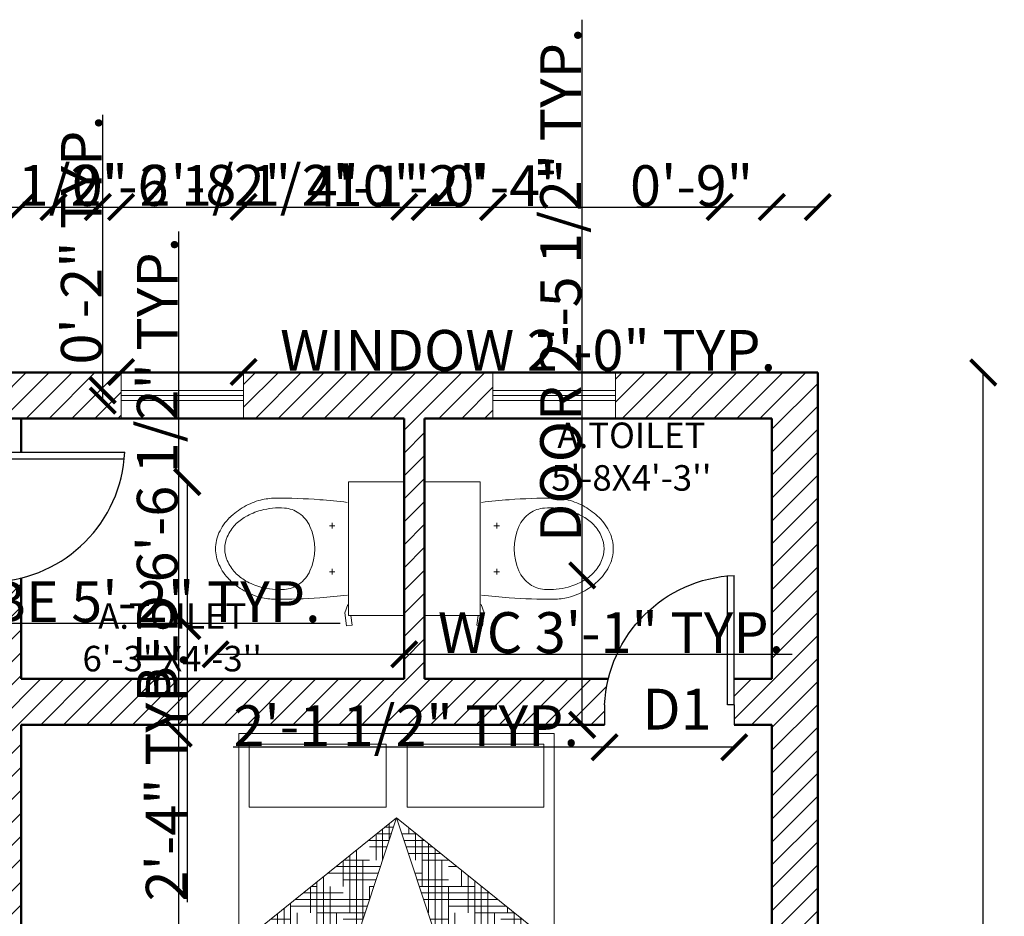
# Model space of a CAD drawing. Units: inches. Extents: x 1385 to 1778, y 1343 to 2100.
# Tile 6 of 6: x 1571 to 1764, y 1924 to 2100. Entities that reach past the tile are written whole.
import ezdxf

# ---------------------------------------------------------------- set-up
doc = ezdxf.new("R2010")
doc.units = ezdxf.units.IN
for name, color, linetype, lineweight in [('A-ANNO-DIMS', 2, 'Continuous', 18), ('A-ANNO-TEXT', 7, 'Continuous', 25), ('A-AREA-IDEN', 7, 'Continuous', 25), ('A-FLOR-FIXT', 9, 'Continuous', 18), ('A-FURN', 8, 'Continuous', 18), ('A-WALL-PATT', 8, 'Continuous', 13), ('Door', 150, 'Continuous', 25), ('Wall', 7, 'Continuous', 50), ('Windows', 140, 'Continuous', 18)]:
    doc.layers.add(name, color=color, linetype=linetype, lineweight=lineweight)
doc.styles.get("Standard").update_dxf_attribs({"font": 'arial.ttf'})
doc.dimstyles.get("Standard").update_dxf_attribs({"dimtxt": 8, "dimasz": 5, "dimexe": 0.18, "dimexo": 0.0625, "dimgap": 0.09, "dimtad": 1, "dimdec": 1, "dimzin": 0, "dimdsep": 46, "dimlunit": 4, "dimtxsty": 'Standard', "dimblk": 'ARCHTICK', "dimcen": 0.09, "dimse1": 1, "dimse2": 1, "dimadec": 0, "dimazin": 0, "dimtfac": 1, "dimtdec": 1, "dimtofl": 0, "dimtmove": 0, "dimatfit": 3, "dimfxl": 1, "dimtolj": 1, "dimtzin": 0, "dimarcsym": 0})

# ---------------------------------------------------------------- blocks, each defined once
blk = doc.blocks.new('AP0B05')
for p, q in [((35, 100), (35, 880)), ((75, 100), (75, 878.9)), ((35, 100), (35, -20)), ((815, 100), (815, -20))]:
    blk.add_line(p, q)
blk.add_lwpolyline([(35, 100), (75, 100)])
blk.add_arc((-2.4, 62.6), 818.3, 2.62122, 87.37878)
blk = doc.blocks.new('toilet-1')
at = {"color": 0, "linetype": 'ByBlock'}
for p, q in [((-0.23, -0.02), (-0.23, -0.2116)), ((0.23, -0.02), (-0.23, -0.02)), ((0.23, -0.02), (0.23, -0.2116)), ((0.2633, -0.1997), (0.23, -0.2044)), ((0.266, -0.2187), (0.2633, -0.1997)), ((-0.23, -0.2116), (0.23, -0.2116)), ((0.1917, -0.2144), (0.2206, -0.225)), ((0.2206, -0.225), (0.266, -0.2187)), ((-0.0889, -0.2683), (-0.0697, -0.2683)), ((-0.0793, -0.2587), (-0.0793, -0.2778)), ((0.0889, -0.2683), (0.0698, -0.2683)), ((0.0794, -0.2587), (0.0794, -0.2778)), ((0, -0.6382), (0, -0.6382))]:
    blk.add_line(p, q, dxfattribs=at)
for centre, radius, start, end in [((3.5272, -0.6239), 3.7093, 173.6925, 175.1593), ((-3.527, -0.624), 3.7093, 4.8413, 6.3171), ((1.7368, -0.4519), 1.9109, 175.7698, 180.3758), ((0, -0.5169), 0.1884, 66.0939, 113.9061), ((-1.7366, -0.4519), 1.9109, 359.6242, 4.2302), ((-0.0312, -0.4465), 0.1114, 113.8997, 145.1485), ((0.0312, -0.4465), 0.1114, 34.8515, 66.1003), ((-0.0408, -0.4398), 0.0996, 145.1497, 175.881), ((0.0409, -0.4398), 0.0996, 4.119, 34.8503), ((0.0981, -0.4497), 0.2389, 175.8862, 195.5931), ((-0.098, -0.4497), 0.2389, 344.4069, 4.1138), ((0.0353, -0.463), 0.2093, 180.3747, 194.3375), ((-0.0351, -0.463), 0.2093, 345.6614, 359.6243), ((0.055, -0.458), 0.2297, 194.3353, 209.622), ((0.0961, -0.4503), 0.2369, 195.5969, 209.3771), ((-0.096, -0.4503), 0.2369, 330.6229, 344.4031), ((-0.0548, -0.458), 0.2297, 330.3788, 345.6655), ((0.0647, -0.4524), 0.2409, 209.6273, 224.5489), ((0.0232, -0.4913), 0.1532, 209.3871, 226.5438), ((-0.0231, -0.4913), 0.1532, 313.4562, 330.6129), ((-0.0645, -0.4524), 0.2409, 315.4504, 330.372), ((0.0152, -0.4997), 0.1416, 226.5501, 246.5527), ((-0.0151, -0.4997), 0.1416, 293.4473, 313.4499), ((0.0178, -0.4986), 0.1751, 224.552, 245.714), ((0, -0.5347), 0.1034, 246.5493, 270.0042), ((0, -0.5347), 0.1034, 269.9958, 293.4507), ((-0.0176, -0.4986), 0.1751, 294.2865, 315.4485), ((0.0004, -0.538), 0.132, 245.5845, 269.8782), ((-0.0002, -0.538), 0.132, 270.1216, 294.4153)]:
    blk.add_arc(centre, radius, start, end, dxfattribs=at)
blk = doc.blocks.new('*X10')
at = {"color": 0}
for p, q in [((20.25, 14.8125), (20.2772, 14.8125)), ((20.1739, 14.75), (20.2772, 14.75)), ((20.1875, 14.75), (20.1875, 14.7669)), ((20.199, 14.7812), (20.2772, 14.7812)), ((20.25, 14.3194), (20.25, 14.75)), ((20.1487, 14.7188), (20.2772, 14.7188)), ((20.1562, 14.625), (20.1562, 14.7281)), ((20.0984, 14.6562), (20.125, 14.6562)), ((20.1236, 14.6875), (20.25, 14.6875)), ((20.125, 14.5), (20.125, 14.6893)), ((20.0625, 14.2573), (20.0625, 14.6116)), ((20.0938, 14.375), (20.0938, 14.6504)), ((20.2188, 14.3091), (20.2188, 14.625)), ((20.25, 14.625), (20.2772, 14.625)), ((20.023, 14.5625), (20.2772, 14.5625)), ((20.0312, 14.2469), (20.0312, 14.5727)), ((20.125, 14.5938), (20.2772, 14.5938)), ((19.9979, 14.5312), (20.2772, 14.5312)), ((19.9476, 14.4688), (20.125, 14.4688)), ((19.9727, 14.5), (20.25, 14.5)), ((20, 14.2366), (20, 14.5)), ((20.1875, 14.2987), (20.1875, 14.5)), ((19.9062, 14.375), (19.9062, 14.4174)), ((19.9225, 14.4375), (20, 14.4375)), ((20.25, 14.4375), (20.2772, 14.4375)), ((19.875, 14.25), (19.875, 14.3785)), ((19.9688, 14.2262), (19.9688, 14.375)), ((20, 14.375), (20.2772, 14.375)), ((20.125, 14.4062), (20.2772, 14.4062)), ((20.1562, 14.2884), (20.1562, 14.375)), ((19.8438, 14.1848), (19.8438, 14.3397)), ((19.875, 14.3438), (20.2772, 14.3438)), ((19.7967, 14.2812), (20.125, 14.2812)), ((19.8125, 14.1744), (19.8125, 14.3008)), ((19.8219, 14.3125), (20.2291, 14.3125)), ((19.7716, 14.25), (20, 14.25)), ((19.7812, 14.1641), (19.7812, 14.262)), ((19.9375, 14.2159), (19.9375, 14.25)), ((19.7213, 14.1875), (19.75, 14.1875)), ((19.7465, 14.2188), (19.875, 14.2188)), ((19.75, 14.1537), (19.75, 14.2231)), ((19.7018, 14.0938), (19.7786, 14.0938)), ((19.7188, 14.0726), (19.7188, 14.1136)), ((19.75, 14.0338), (19.75, 14.1032)), ((19.7812, 13.9949), (19.7812, 14.0929)), ((19.7269, 14.0625), (19.8728, 14.0625)), ((19.8125, 14), (19.8125, 14.0825)), ((19.9062, 13.8396), (19.9062, 14.0514)), ((19.752, 14.0312), (19.875, 14.0312)), ((19.875, 13.8784), (19.875, 14)), ((19.9375, 13.8007), (19.9375, 14.0411)), ((19.9688, 13.875), (19.9688, 14.0307)), ((20, 14), (20, 14.0204)), ((20, 14), (20.0614, 14)), ((20.0625, 13.6454), (20.0625, 13.9996)), ((19.875, 13.9688), (20.1557, 13.9688)), ((20.0938, 13.625), (20.0938, 13.9893)), ((20.125, 13.75), (20.125, 13.9789)), ((20.1562, 13.875), (20.1562, 13.9686)), ((19.8275, 13.9375), (20.25, 13.9375)), ((19.8526, 13.9062), (20.125, 13.9062)), ((20.25, 13.5), (20.25, 13.9375)), ((19.8777, 13.875), (20, 13.875)), ((20.0312, 13.6842), (20.0312, 13.875)), ((20.2188, 13.4511), (20.2188, 13.875)), ((20.25, 13.875), (20.2772, 13.875)), ((20, 13.8125), (20.2772, 13.8125)), ((20.125, 13.8438), (20.2772, 13.8438)), ((19.9532, 13.7812), (20.2772, 13.7812)), ((19.9783, 13.75), (20.25, 13.75)), ((20, 13.723), (20, 13.75)), ((20.0035, 13.7188), (20.125, 13.7188)), ((20.1875, 13.49), (20.1875, 13.75)), ((20.25, 13.6875), (20.2772, 13.6875)), ((20.0789, 13.625), (20.2772, 13.625)), ((20.125, 13.6562), (20.2772, 13.6562)), ((20.1562, 13.5288), (20.1562, 13.625)), ((20.104, 13.5938), (20.2772, 13.5938)), ((20.1292, 13.5625), (20.25, 13.5625)), ((20.25, 13.5), (20.2772, 13.5)), ((20.2046, 13.4688), (20.2772, 13.4688)), ((20.2297, 13.4375), (20.2772, 13.4375)), ((20.2549, 13.4062), (20.2772, 13.4062))]:
    blk.add_line(p, q, dxfattribs=at)
blk = doc.blocks.new('MAT-P13')
for p, q in [((-0.75, 0), (0.75, 0)), ((-0.75, 0), (-0.75, -1.9)), ((0.75, 0), (0.75, -1.9)), ((-0.7, -0.05), (-0.7, -0.35)), ((-0.7, -0.05), (-0.05, -0.05)), ((-0.05, -0.35), (-0.05, -0.05)), ((0.05, -0.05), (0.7, -0.05)), ((0.05, -0.35), (0.05, -0.05)), ((0.7, -0.05), (0.7, -0.35)), ((-0.7, -0.35), (-0.05, -0.35)), ((0.05, -0.35), (0.7, -0.35)), ((-0.75, -1.0034), (0, -0.4)), ((0, -0.4), (-0.75, -1.0034)), ((0, -0.4), (-0.2, -1.0034)), ((0, -0.4), (0.2, -1.0034)), ((0, -0.4), (0.75, -1.0034)), ((-0.75, -1.0034), (-0.2, -1.0034)), ((0.2, -1.0034), (0.75, -1.0034)), ((0.75, -1.9), (-0.75, -1.9))]:
    blk.add_line(p, q)
at = {"xscale": -1, "rotation": 90}
blk.add_blockref('*X10', (14.1285, 19.2738), dxfattribs=at)
blk = doc.blocks.new('WINDOW-GLAZING-24IN')
for p, q in [((0, 2), (24, 2)), ((0, 1), (24, 1)), ((0, 0), (24, 0))]:
    blk.add_line(p, q)
blk = doc.blocks.new('_ArchTick')
at = {"color": 0, "linetype": 'ByBlock', "const_width": 0.15}
blk.add_lwpolyline([(-0.5, -0.5), (0.5, 0.5)], dxfattribs=at)
blk = doc.blocks.new('*D17')
at = {"layer": 'A-ANNO-DIMS', "color": 0, "lineweight": -2, "transparency": 16777216}
for p, q in [((1681.63, 1991), (1681.63, 2099.82)), ((1681.63, 1961.73), (1681.63, 1991))]:
    blk.add_line(p, q, dxfattribs=at)
at = {"layer": 'Defpoints', "color": 0, "transparency": 16777216}
for p in [(1681.63, 1991), (1686.02, 1991), (1686.02, 1961.73)]:
    blk.add_point(p, dxfattribs=at)
at = {"layer": 'A-ANNO-DIMS', "color": 0, "lineweight": -2, "transparency": 16777216, "xscale": 5, "yscale": 5, "zscale": 5}
for p, rotation in [((1681.63, 1991), 90), ((1681.63, 1961.73), 270)]:
    blk.add_blockref('_ArchTick', p, dxfattribs=dict(at, rotation=rotation))
at = {"layer": 'A-ANNO-DIMS', "color": 0, "transparency": 16777216, "insert": (1677.4, 2047.91), "char_height": 8, "attachment_point": 5, "rotation": 90}
blk.add_mtext('\\A1;DOOR 2\'-5 1/2" TYP.', dxfattribs=at)
blk = doc.blocks.new('*D18')
at = {"layer": 'A-ANNO-DIMS', "color": 0, "lineweight": -2, "transparency": 16777216}
for p, q in [((1686.02, 1957.34), (1613.3, 1957.34)), ((1711.39, 1957.34), (1686.02, 1957.34))]:
    blk.add_line(p, q, dxfattribs=at)
at = {"layer": 'Defpoints', "color": 0, "transparency": 16777216}
for p in [(1686.02, 1961.73), (1711.39, 1961.73), (1686.02, 1957.34)]:
    blk.add_point(p, dxfattribs=at)
at = {"layer": 'A-ANNO-DIMS', "color": 0, "lineweight": -2, "transparency": 16777216, "xscale": 5, "yscale": 5, "zscale": 5, "rotation": 180}
blk.add_blockref('_ArchTick', (1686.02, 1957.34), dxfattribs=at)
at = {"layer": 'A-ANNO-DIMS', "color": 0, "lineweight": -2, "transparency": 16777216, "xscale": 5, "yscale": 5, "zscale": 5}
blk.add_blockref('_ArchTick', (1711.39, 1957.34), dxfattribs=at)
at = {"layer": 'A-ANNO-DIMS', "color": 0, "transparency": 16777216, "insert": (1647.16, 1961.57), "char_height": 8, "attachment_point": 5}
blk.add_mtext('\\A1;2\'-1 1/2" TYP.', dxfattribs=at)
blk = doc.blocks.new('*D29')
at = {"layer": 'A-ANNO-DIMS', "color": 0, "lineweight": -2, "transparency": 16777216}
for p, q in [((1591.32, 2030.83), (1615.32, 2030.83)), ((1615.32, 2030.83), (1721.74, 2030.83))]:
    blk.add_line(p, q, dxfattribs=at)
at = {"layer": 'Defpoints', "color": 0, "transparency": 16777216}
for p in [(1615.32, 2030.83), (1591.32, 2027.23), (1615.32, 2027.23)]:
    blk.add_point(p, dxfattribs=at)
at = {"layer": 'A-ANNO-DIMS', "color": 0, "lineweight": -2, "transparency": 16777216, "xscale": 5, "yscale": 5, "zscale": 5, "rotation": 180}
blk.add_blockref('_ArchTick', (1591.32, 2030.83), dxfattribs=at)
at = {"layer": 'A-ANNO-DIMS', "color": 0, "lineweight": -2, "transparency": 16777216, "xscale": 5, "yscale": 5, "zscale": 5}
blk.add_blockref('_ArchTick', (1615.32, 2030.83), dxfattribs=at)
at = {"layer": 'A-ANNO-DIMS', "color": 0, "transparency": 16777216, "insert": (1671.03, 2035.06), "char_height": 8, "attachment_point": 5}
blk.add_mtext('\\A1;WINDOW 2\'-0" TYP.', dxfattribs=at)
blk = doc.blocks.new('*D30')
at = {"layer": 'A-ANNO-DIMS', "color": 0, "lineweight": -2, "transparency": 16777216}
for p, q in [((1587.72, 2027.23), (1587.72, 2081.18)), ((1587.72, 2025.23), (1587.72, 2027.23))]:
    blk.add_line(p, q, dxfattribs=at)
at = {"layer": 'Defpoints', "color": 0, "transparency": 16777216}
for p in [(1587.72, 2027.23), (1591.32, 2027.23), (1591.32, 2025.23)]:
    blk.add_point(p, dxfattribs=at)
at = {"layer": 'A-ANNO-DIMS', "color": 0, "lineweight": -2, "transparency": 16777216, "xscale": 5, "yscale": 5, "zscale": 5}
for p, rotation in [((1587.72, 2027.23), 90), ((1587.72, 2025.23), 270)]:
    blk.add_blockref('_ArchTick', p, dxfattribs=dict(at, rotation=rotation))
at = {"layer": 'A-ANNO-DIMS', "color": 0, "transparency": 16777216, "insert": (1583.55, 2056.71), "char_height": 8, "attachment_point": 5, "rotation": 90}
blk.add_mtext('\\A1;0\'-2" TYP.', dxfattribs=at)
blk = doc.blocks.new('*D33')
at = {"layer": 'A-ANNO-DIMS', "color": 0, "lineweight": -2, "transparency": 16777216}
for p, q in [((1609.83, 1975.57), (1646.77, 1975.57)), ((1646.77, 1975.57), (1722.77, 1975.57))]:
    blk.add_line(p, q, dxfattribs=at)
at = {"layer": 'Defpoints', "color": 0, "transparency": 16777216}
for p in [(1609.83, 1981.11), (1646.77, 1981.11), (1646.77, 1975.57)]:
    blk.add_point(p, dxfattribs=at)
at = {"layer": 'A-ANNO-DIMS', "color": 0, "lineweight": -2, "transparency": 16777216, "xscale": 5, "yscale": 5, "zscale": 5, "rotation": 180}
blk.add_blockref('_ArchTick', (1609.83, 1975.57), dxfattribs=at)
at = {"layer": 'A-ANNO-DIMS', "color": 0, "lineweight": -2, "transparency": 16777216, "xscale": 5, "yscale": 5, "zscale": 5}
blk.add_blockref('_ArchTick', (1646.77, 1975.57), dxfattribs=at)
at = {"layer": 'A-ANNO-DIMS', "color": 0, "transparency": 16777216, "insert": (1687.27, 1979.8), "char_height": 8, "attachment_point": 5}
blk.add_mtext('\\A1;WC 3\'-1" TYP.', dxfattribs=at)
blk = doc.blocks.new('*D34')
at = {"layer": 'A-ANNO-DIMS', "color": 0, "lineweight": -2, "transparency": 16777216}
for p, q in [((1604.28, 2009.31), (1604.28, 1981.11)), ((1604.28, 1981.11), (1604.28, 1927.03))]:
    blk.add_line(p, q, dxfattribs=at)
at = {"layer": 'Defpoints', "color": 0, "transparency": 16777216}
for p in [(1609.83, 2009.31), (1604.28, 1981.11), (1609.83, 1981.11)]:
    blk.add_point(p, dxfattribs=at)
at = {"layer": 'A-ANNO-DIMS', "color": 0, "lineweight": -2, "transparency": 16777216, "xscale": 5, "yscale": 5, "zscale": 5}
for p, rotation in [((1604.28, 2009.31), 90), ((1604.28, 1981.11), 270)]:
    blk.add_blockref('_ArchTick', p, dxfattribs=dict(at, rotation=rotation))
at = {"layer": 'A-ANNO-DIMS', "color": 0, "transparency": 16777216, "insert": (1600.17, 1951.57), "char_height": 8, "attachment_point": 5, "rotation": 90}
blk.add_mtext('\\A1;2\'-4" TYP.', dxfattribs=at)
blk = doc.blocks.new('*D35')
at = {"layer": 'A-ANNO-DIMS', "color": 0, "lineweight": -2, "transparency": 16777216}
for p, q in [((1602.63, 1960.02), (1602.63, 2058.34)), ((1602.63, 1881.75), (1602.63, 1960.02))]:
    blk.add_line(p, q, dxfattribs=at)
at = {"layer": 'Defpoints', "color": 0, "transparency": 16777216}
for p in [(1602.63, 1960.02), (1614.37, 1960.02), (1614.37, 1881.75)]:
    blk.add_point(p, dxfattribs=at)
at = {"layer": 'A-ANNO-DIMS', "color": 0, "lineweight": -2, "transparency": 16777216, "xscale": 5, "yscale": 5, "zscale": 5}
for p, rotation in [((1602.63, 1960.02), 90), ((1602.63, 1881.75), 270)]:
    blk.add_blockref('_ArchTick', p, dxfattribs=dict(at, rotation=rotation))
at = {"layer": 'A-ANNO-DIMS', "color": 0, "transparency": 16777216, "insert": (1598.41, 2011.68), "char_height": 8, "attachment_point": 5, "rotation": 90}
blk.add_mtext('\\A1;BED 6\'-6 1/2" TYP.', dxfattribs=at)
blk = doc.blocks.new('*D37')
at = {"layer": 'A-ANNO-DIMS', "color": 0, "lineweight": -2, "transparency": 16777216}
for p, q in [((1449.17, 1981.63), (1511.01, 1981.63)), ((1511.01, 1981.63), (1634.21, 1981.63))]:
    blk.add_line(p, q, dxfattribs=at)
at = {"layer": 'Defpoints', "color": 0, "transparency": 16777216}
for p in [(1449.17, 1990.9), (1511.01, 1990.9), (1511.01, 1981.63)]:
    blk.add_point(p, dxfattribs=at)
at = {"layer": 'A-ANNO-DIMS', "color": 0, "lineweight": -2, "transparency": 16777216, "xscale": 5, "yscale": 5, "zscale": 5, "rotation": 180}
blk.add_blockref('_ArchTick', (1449.17, 1981.63), dxfattribs=at)
at = {"layer": 'A-ANNO-DIMS', "color": 0, "lineweight": -2, "transparency": 16777216, "xscale": 5, "yscale": 5, "zscale": 5}
blk.add_blockref('_ArchTick', (1511.01, 1981.63), dxfattribs=at)
at = {"layer": 'A-ANNO-DIMS', "color": 0, "transparency": 16777216, "insert": (1575.11, 1985.86), "char_height": 8, "attachment_point": 5}
blk.add_mtext('\\A1;WARDROBE 5\'-2" TYP.', dxfattribs=at)
blk = doc.blocks.new('*D50')
at = {"layer": 'A-ANNO-DIMS', "color": 0, "lineweight": -2, "transparency": 16777216}
blk.add_line((1760.18, 1382.73), (1760.18, 2030.73), dxfattribs=at)
at = {"layer": 'Defpoints', "color": 0, "transparency": 16777216}
for p in [(1727.77, 2030.73), (1760.18, 2030.73), (1727.77, 1382.73)]:
    blk.add_point(p, dxfattribs=at)
at = {"layer": 'A-ANNO-DIMS', "color": 0, "lineweight": -2, "transparency": 16777216, "xscale": 5, "yscale": 5, "zscale": 5}
for p, rotation in [((1760.18, 2030.73), 90), ((1760.18, 1382.73), 270)]:
    blk.add_blockref('_ArchTick', p, dxfattribs=dict(at, rotation=rotation))
at = {"layer": 'A-ANNO-DIMS', "color": 0, "transparency": 16777216, "insert": (1756, 1706.73), "char_height": 8, "attachment_point": 5, "rotation": 90}
blk.add_mtext('\\A1;54\'-0"', dxfattribs=at)
blk = doc.blocks.new('*D52')
at = {"layer": 'A-ANNO-DIMS', "color": 0, "lineweight": -2, "transparency": 16777216}
for p, q in [((1558.75, 2063.14), (1591.32, 2063.14)), ((1591.32, 2063.14), (1636.55, 2063.14))]:
    blk.add_line(p, q, dxfattribs=at)
at = {"layer": 'Defpoints', "color": 0, "transparency": 16777216}
for p in [(1591.32, 2063.14), (1558.75, 2030.73), (1591.32, 2030.73)]:
    blk.add_point(p, dxfattribs=at)
at = {"layer": 'A-ANNO-DIMS', "color": 0, "lineweight": -2, "transparency": 16777216, "xscale": 5, "yscale": 5, "zscale": 5, "rotation": 180}
blk.add_blockref('_ArchTick', (1558.75, 2063.14), dxfattribs=at)
at = {"layer": 'A-ANNO-DIMS', "color": 0, "lineweight": -2, "transparency": 16777216, "xscale": 5, "yscale": 5, "zscale": 5}
blk.add_blockref('_ArchTick', (1591.32, 2063.14), dxfattribs=at)
at = {"layer": 'A-ANNO-DIMS', "color": 0, "transparency": 16777216, "insert": (1616.44, 2067.37), "char_height": 8, "attachment_point": 5}
blk.add_mtext('\\A1;2\'-8 1/2"', dxfattribs=at)
blk = doc.blocks.new('*D53')
at = {"layer": 'A-ANNO-DIMS', "color": 0, "lineweight": -2, "transparency": 16777216}
blk.add_line((1615.32, 2063.14), (1664.16, 2063.14), dxfattribs=at)
at = {"layer": 'Defpoints', "color": 0, "transparency": 16777216}
for p in [(1664.16, 2063.14), (1615.32, 2030.73), (1664.16, 2030.73)]:
    blk.add_point(p, dxfattribs=at)
at = {"layer": 'A-ANNO-DIMS', "color": 0, "lineweight": -2, "transparency": 16777216, "xscale": 5, "yscale": 5, "zscale": 5, "rotation": 180}
blk.add_blockref('_ArchTick', (1615.32, 2063.14), dxfattribs=at)
at = {"layer": 'A-ANNO-DIMS', "color": 0, "lineweight": -2, "transparency": 16777216, "xscale": 5, "yscale": 5, "zscale": 5}
blk.add_blockref('_ArchTick', (1664.16, 2063.14), dxfattribs=at)
at = {"layer": 'A-ANNO-DIMS', "color": 0, "transparency": 16777216, "insert": (1639.74, 2067.25), "char_height": 8, "attachment_point": 5}
blk.add_mtext('\\A1;4\'-1"', dxfattribs=at)
blk = doc.blocks.new('*D54')
at = {"layer": 'A-ANNO-DIMS', "color": 0, "lineweight": -2, "transparency": 16777216}
blk.add_line((1401.37, 1961.73), (1401.37, 1904.94), dxfattribs=at)
at = {"layer": 'Defpoints', "color": 0, "transparency": 16777216}
for p in [(1718.77, 1961.73), (1401.37, 1904.94), (1718.77, 1904.94)]:
    blk.add_point(p, dxfattribs=at)
at = {"layer": 'A-ANNO-DIMS', "color": 0, "lineweight": -2, "transparency": 16777216, "xscale": 5, "yscale": 5, "zscale": 5}
for p, rotation in [((1401.37, 1961.73), 90), ((1401.37, 1904.94), 270)]:
    blk.add_blockref('_ArchTick', p, dxfattribs=dict(at, rotation=rotation))
at = {"layer": 'A-ANNO-DIMS', "color": 0, "transparency": 16777216, "insert": (1397.19, 1933.34), "char_height": 8, "attachment_point": 5, "rotation": 90}
blk.add_mtext('\\A1;4\'-9"', dxfattribs=at)
blk = doc.blocks.new('*D61')
at = {"layer": 'A-ANNO-DIMS', "color": 0, "lineweight": -2, "transparency": 16777216}
blk.add_line((1586.77, 2063.14), (1708.55, 2063.14), dxfattribs=at)
at = {"layer": 'Defpoints', "color": 0, "transparency": 16777216}
for p in [(1708.55, 2063.14), (1586.77, 1382.73), (1708.55, 1382.73)]:
    blk.add_point(p, dxfattribs=at)
at = {"layer": 'A-ANNO-DIMS', "color": 0, "lineweight": -2, "transparency": 16777216, "xscale": 5, "yscale": 5, "zscale": 5, "rotation": 180}
blk.add_blockref('_ArchTick', (1586.77, 2063.14), dxfattribs=at)
at = {"layer": 'A-ANNO-DIMS', "color": 0, "lineweight": -2, "transparency": 16777216, "xscale": 5, "yscale": 5, "zscale": 5}
blk.add_blockref('_ArchTick', (1708.55, 2063.14), dxfattribs=at)
at = {"layer": 'A-ANNO-DIMS', "color": 0, "transparency": 16777216, "insert": (1647.66, 2067.31), "char_height": 8, "attachment_point": 5}
blk.add_mtext('\\A1;10\'-2"', dxfattribs=at)
blk = doc.blocks.new('*D67')
at = {"layer": 'A-ANNO-DIMS', "color": 0, "lineweight": -2, "transparency": 16777216}
for p, q in [((1513.34, 2063.14), (1546.08, 2063.14)), ((1546.08, 2063.14), (1591.31, 2063.14))]:
    blk.add_line(p, q, dxfattribs=at)
at = {"layer": 'Defpoints', "color": 0, "transparency": 16777216}
for p in [(1546.08, 2063.14), (1513.34, 1595.73), (1546.08, 1595.73)]:
    blk.add_point(p, dxfattribs=at)
at = {"layer": 'A-ANNO-DIMS', "color": 0, "lineweight": -2, "transparency": 16777216, "xscale": 5, "yscale": 5, "zscale": 5, "rotation": 180}
blk.add_blockref('_ArchTick', (1513.34, 2063.14), dxfattribs=at)
at = {"layer": 'A-ANNO-DIMS', "color": 0, "lineweight": -2, "transparency": 16777216, "xscale": 5, "yscale": 5, "zscale": 5}
blk.add_blockref('_ArchTick', (1546.08, 2063.14), dxfattribs=at)
at = {"layer": 'A-ANNO-DIMS', "color": 0, "transparency": 16777216, "insert": (1571.19, 2067.37), "char_height": 8, "attachment_point": 5}
blk.add_mtext('\\A1;2\'-8 1/2"', dxfattribs=at)
blk = doc.blocks.new('*D70')
at = {"layer": 'A-ANNO-DIMS', "color": 0, "lineweight": -2, "transparency": 16777216}
for p, q in [((1571.77, 2063.14), (1578.09, 2063.14)), ((1578.09, 2063.14), (1623.18, 2063.14))]:
    blk.add_line(p, q, dxfattribs=at)
at = {"layer": 'Defpoints', "color": 0, "transparency": 16777216}
for p in [(1578.09, 2063.14), (1571.77, 1829.73), (1578.09, 1829.73)]:
    blk.add_point(p, dxfattribs=at)
at = {"layer": 'A-ANNO-DIMS', "color": 0, "lineweight": -2, "transparency": 16777216, "xscale": 5, "yscale": 5, "zscale": 5, "rotation": 180}
blk.add_blockref('_ArchTick', (1571.77, 2063.14), dxfattribs=at)
at = {"layer": 'A-ANNO-DIMS', "color": 0, "lineweight": -2, "transparency": 16777216, "xscale": 5, "yscale": 5, "zscale": 5}
blk.add_blockref('_ArchTick', (1578.09, 2063.14), dxfattribs=at)
at = {"layer": 'A-ANNO-DIMS', "color": 0, "transparency": 16777216, "insert": (1603.14, 2067.37), "char_height": 8, "attachment_point": 5}
blk.add_mtext('\\A1;0\'-6 1/2"', dxfattribs=at)
blk = doc.blocks.new('*D71')
at = {"layer": 'A-ANNO-DIMS', "color": 0, "lineweight": -2, "transparency": 16777216}
for p, q in [((1646.77, 2063.14), (1650.77, 2063.14)), ((1650.77, 2063.14), (1677.22, 2063.14))]:
    blk.add_line(p, q, dxfattribs=at)
at = {"layer": 'Defpoints', "color": 0, "transparency": 16777216}
for p in [(1650.77, 2063.14), (1646.77, 2021.73), (1650.77, 2021.73)]:
    blk.add_point(p, dxfattribs=at)
at = {"layer": 'A-ANNO-DIMS', "color": 0, "lineweight": -2, "transparency": 16777216, "xscale": 5, "yscale": 5, "zscale": 5, "rotation": 180}
blk.add_blockref('_ArchTick', (1646.77, 2063.14), dxfattribs=at)
at = {"layer": 'A-ANNO-DIMS', "color": 0, "lineweight": -2, "transparency": 16777216, "xscale": 5, "yscale": 5, "zscale": 5}
blk.add_blockref('_ArchTick', (1650.77, 2063.14), dxfattribs=at)
at = {"layer": 'A-ANNO-DIMS', "color": 0, "transparency": 16777216, "insert": (1666.5, 2067.31), "char_height": 8, "attachment_point": 5}
blk.add_mtext('\\A1;0\'-4"', dxfattribs=at)
blk = doc.blocks.new('*D72')
at = {"layer": 'A-ANNO-DIMS', "color": 0, "lineweight": -2, "transparency": 16777216}
for p, q in [((1718.77, 2063.14), (1692.33, 2063.14)), ((1727.77, 2063.14), (1718.77, 2063.14))]:
    blk.add_line(p, q, dxfattribs=at)
at = {"layer": 'Defpoints', "color": 0, "transparency": 16777216}
for p in [(1718.77, 2063.14), (1727.77, 2030.73), (1718.77, 2021.73)]:
    blk.add_point(p, dxfattribs=at)
at = {"layer": 'A-ANNO-DIMS', "color": 0, "lineweight": -2, "transparency": 16777216, "xscale": 5, "yscale": 5, "zscale": 5, "rotation": 180}
blk.add_blockref('_ArchTick', (1718.77, 2063.14), dxfattribs=at)
at = {"layer": 'A-ANNO-DIMS', "color": 0, "lineweight": -2, "transparency": 16777216, "xscale": 5, "yscale": 5, "zscale": 5}
blk.add_blockref('_ArchTick', (1727.77, 2063.14), dxfattribs=at)
at = {"layer": 'A-ANNO-DIMS', "color": 0, "transparency": 16777216, "insert": (1703.05, 2067.31), "char_height": 8, "attachment_point": 5}
blk.add_mtext('\\A1;0\'-9"', dxfattribs=at)
blk = doc.blocks.new('*D75')
at = {"layer": 'A-ANNO-DIMS', "color": 0, "lineweight": -2, "transparency": 16777216}
for p, q in [((1401.37, 2021.73), (1401.37, 2066.82)), ((1401.37, 2015.14), (1401.37, 2021.73))]:
    blk.add_line(p, q, dxfattribs=at)
at = {"layer": 'Defpoints', "color": 0, "transparency": 16777216}
for p in [(1401.37, 2021.73), (1571.77, 2021.73), (1571.77, 2015.14)]:
    blk.add_point(p, dxfattribs=at)
at = {"layer": 'A-ANNO-DIMS', "color": 0, "lineweight": -2, "transparency": 16777216, "xscale": 5, "yscale": 5, "zscale": 5}
for p, rotation in [((1401.37, 2021.73), 90), ((1401.37, 2015.14), 270)]:
    blk.add_blockref('_ArchTick', p, dxfattribs=dict(at, rotation=rotation))
at = {"layer": 'A-ANNO-DIMS', "color": 0, "transparency": 16777216, "insert": (1397.14, 2046.78), "char_height": 8, "attachment_point": 5, "rotation": 90}
blk.add_mtext('\\A1;0\'-6 1/2"', dxfattribs=at)
blk = doc.blocks.new('*D76')
at = {"layer": 'A-ANNO-DIMS', "color": 0, "lineweight": -2, "transparency": 16777216}
for p, q in [((1711.39, 1350.33), (1718.77, 1350.33)), ((1718.77, 1350.33), (1763.86, 1350.33))]:
    blk.add_line(p, q, dxfattribs=at)
at = {"layer": 'Defpoints', "color": 0, "transparency": 16777216}
for p in [(1711.39, 1970.73), (1718.77, 1970.73), (1718.77, 1350.33)]:
    blk.add_point(p, dxfattribs=at)
at = {"layer": 'A-ANNO-DIMS', "color": 0, "lineweight": -2, "transparency": 16777216, "xscale": 5, "yscale": 5, "zscale": 5, "rotation": 180}
blk.add_blockref('_ArchTick', (1711.39, 1350.33), dxfattribs=at)
at = {"layer": 'A-ANNO-DIMS', "color": 0, "lineweight": -2, "transparency": 16777216, "xscale": 5, "yscale": 5, "zscale": 5}
blk.add_blockref('_ArchTick', (1718.77, 1350.33), dxfattribs=at)
at = {"layer": 'A-ANNO-DIMS', "color": 0, "transparency": 16777216, "insert": (1743.82, 1354.56), "char_height": 8, "attachment_point": 5}
blk.add_mtext('\\A1;0\'-7 1/2"', dxfattribs=at)
blk = doc.blocks.new('*D82')
at = {"layer": 'A-ANNO-DIMS', "color": 0, "lineweight": -2, "transparency": 16777216}
for p, q in [((1401.37, 2021.73), (1401.37, 2009.31)), ((1401.37, 2009.31), (1401.37, 1964.97))]:
    blk.add_line(p, q, dxfattribs=at)
at = {"layer": 'Defpoints', "color": 0, "transparency": 16777216}
for p in [(1646.77, 2021.73), (1401.37, 2009.31), (1646.77, 2009.31)]:
    blk.add_point(p, dxfattribs=at)
at = {"layer": 'A-ANNO-DIMS', "color": 0, "lineweight": -2, "transparency": 16777216, "xscale": 5, "yscale": 5, "zscale": 5}
for p, rotation in [((1401.37, 2021.73), 90), ((1401.37, 2009.31), 270)]:
    blk.add_blockref('_ArchTick', p, dxfattribs=dict(at, rotation=rotation))
at = {"layer": 'A-ANNO-DIMS', "color": 0, "transparency": 16777216, "insert": (1397.14, 1984.64), "char_height": 8, "attachment_point": 5, "rotation": 90}
blk.add_mtext('\\A1;1\'-0 1/2"', dxfattribs=at)

msp = doc.modelspace()

# ---------------------------------------------------------------- hatches: boundary and pattern name
at = {"layer": 'A-WALL-PATT', "transparency": 33554585}
h = msp.add_hatch(dxfattribs=at)
h.set_pattern_fill('ANSI31', color=256)
h.paths.add_polyline_path([(1522.75, 2030.73), (1433.77, 2030.73), (1433.77, 1900.6), (1442.77, 1900.6), (1442.77, 2021.73), (1522.75, 2021.73)])
h.paths.add_polyline_path([(1591.32, 2030.73), (1558.75, 2030.73), (1558.75, 2021.73), (1571.77, 2021.73), (1591.32, 2021.73)], flags=17)
h.paths.add_polyline_path([(1664.16, 2030.73), (1615.32, 2030.73), (1615.32, 2021.73), (1646.77, 2021.73), (1646.77, 1970.73), (1571.77, 1970.73), (1571.77, 1990.51, -0.048507), (1566.67, 1989.78), (1562.77, 1989.78), (1562.77, 1829.73), (1557.76, 1829.73), (1557.76, 1826.48), (1557.76, 1820.73), (1578.09, 1820.73), (1578.09, 1825.8), (1578.09, 1829.73), (1571.77, 1829.73), (1571.77, 1961.73), (1686.02, 1961.73), (1686.02, 1965.64, -0.048507), (1686.76, 1970.73), (1650.77, 1970.73), (1650.77, 2021.73), (1664.16, 2021.73)])
h.paths.add_polyline_path([(1727.77, 2030.73), (1688.16, 2030.73), (1688.16, 2021.73), (1718.77, 2021.73), (1718.77, 1970.73), (1711.39, 1970.73), (1711.39, 1965.64), (1711.39, 1961.73), (1718.77, 1961.73), (1718.77, 1904.94), (1727.77, 1904.94)])
h.paths.add_polyline_path([(1727.77, 1868.94), (1718.77, 1868.94), (1718.77, 1829.73), (1610.61, 1829.73, -0.028655), (1611.02, 1825.8), (1611.02, 1820.73), (1718.77, 1820.73), (1718.77, 1742.73), (1727.77, 1742.73)])
h.paths.add_polyline_path([(1520.45, 1826.48, -0.020905), (1520.74, 1829.73), (1442.77, 1829.73), (1442.77, 1840.6), (1433.77, 1840.6), (1433.77, 1794.33), (1442.77, 1794.33), (1442.77, 1820.73), (1502.77, 1820.73), (1502.77, 1760.73), (1497.07, 1760.73), (1497.07, 1759.8), (1497.07, 1754.73), (1508.77, 1754.73), (1508.77, 1778.73), (1562.77, 1778.73), (1562.77, 1656.82), (1571.77, 1656.82), (1571.77, 1784.73), (1508.77, 1784.73), (1508.77, 1820.73), (1520.45, 1820.73)])
h.paths.add_polyline_path([(1442.77, 1770.33), (1433.77, 1770.33), (1433.77, 1683.46), (1442.77, 1683.46)], flags=17)
h.paths.add_polyline_path([(1656.16, 1603.19, -0.007591), (1656.26, 1604.73), (1622.77, 1604.73), (1622.77, 1595.73), (1656.16, 1595.73)])
h.paths.add_polyline_path([(1727.77, 1682.73), (1718.77, 1682.73), (1718.77, 1604.73), (1704.65, 1604.73), (1704.65, 1603.19), (1704.65, 1595.73), (1727.77, 1595.73)])
h.paths.add_polyline_path([(1513.34, 1595.73), (1513.34, 1604.73), (1442.77, 1604.73), (1442.77, 1647.46), (1433.77, 1647.46), (1433.77, 1531.33), (1442.77, 1531.33), (1442.77, 1595.73)])
h.paths.add_polyline_path([(1546.08, 1604.73), (1546.08, 1595.73), (1577.77, 1595.73), (1577.77, 1472.73), (1541.77, 1472.73), (1541.77, 1523.73), (1537.77, 1523.73), (1537.77, 1472.73), (1442.77, 1472.73), (1442.77, 1495.33), (1433.77, 1495.33), (1433.77, 1382.73), (1586.77, 1382.73), (1586.77, 1391.73), (1442.77, 1391.73), (1442.77, 1463.73), (1586.77, 1463.73), (1586.77, 1604.73)])

# ---------------------------------------------------------------- linework, layer by layer
at = {"layer": 'Wall'}
for p, q in [((1433.77, 2030.73), (1727.77, 2030.73)), ((1727.77, 2030.73), (1727.77, 1595.73)), ((1442.77, 2021.73), (1571.77, 2021.73)), ((1571.77, 2021.73), (1571.77, 2015.14)), ((1571.77, 2021.73), (1646.77, 2021.73)), ((1646.77, 2021.73), (1646.77, 1970.73)), ((1650.77, 2021.73), (1650.77, 1970.73)), ((1650.77, 2021.73), (1718.77, 2021.73)), ((1718.77, 2021.73), (1718.77, 1970.73)), ((1571.77, 1990.51), (1571.77, 1970.73)), ((1571.77, 1970.73), (1646.77, 1970.73)), ((1650.77, 1970.73), (1686.76, 1970.73)), ((1711.39, 1970.73), (1718.77, 1970.73)), ((1571.77, 1961.73), (1686.02, 1961.73)), ((1571.77, 1961.73), (1571.77, 1829.73)), ((1711.39, 1961.73), (1718.77, 1961.73)), ((1718.77, 1961.73), (1718.77, 1829.73))]:
    msp.add_line(p, q, dxfattribs=at)
at = {"layer": 'Windows'}
for points in [[(1591.32, 2030.73), (1615.32, 2030.73), (1615.32, 2021.73), (1591.32, 2021.73)], [(1664.16, 2030.73), (1688.16, 2030.73), (1688.16, 2021.73), (1664.16, 2021.73)]]:
    msp.add_lwpolyline(points, close=True, dxfattribs=at)

# ---------------------------------------------------------------- block references
at = {"layer": 'A-FLOR-FIXT', "yscale": 56.8416917898501, "zscale": 56.8416917898501}
for p, xscale, rotation in [((1647.91, 1996.23), 56.8416917898501, 270), ((1649.64, 1996.23), -56.8416917898501, 90)]:
    msp.add_blockref('toilet-1', p, dxfattribs=dict(at, xscale=xscale, rotation=rotation))
at = {"layer": 'A-FURN', "xscale": -41.19665858361839, "yscale": 41.19665858361839, "zscale": 41.19665858361839}
msp.add_blockref('MAT-P13', (1645.27, 1960.02), dxfattribs=at)
at = {"layer": 'Door', "xscale": 0.0325161801220908, "yscale": 0.0325161801220908, "zscale": 0.0325161801220908, "rotation": 270}
msp.add_blockref('AP0B05', (1563.42, 2016.28), dxfattribs=at)
at = {"layer": 'Door', "xscale": -0.0325161801220908, "yscale": 0.0325161801220908, "zscale": 0.0325161801220908}
msp.add_blockref('AP0B05', (1712.52, 1962.38), dxfattribs=at)
at = {"layer": 'Windows'}
for p in [(1591.32, 2025.23), (1664.16, 2025.23)]:
    msp.add_blockref('WINDOW-GLAZING-24IN', p, dxfattribs=at)

# ---------------------------------------------------------------- texts
at = {"layer": 'A-ANNO-TEXT'}
msp.add_text('D1', height=8, dxfattribs=at).set_placement((1693.4, 1960.81))
at = {"layer": 'A-AREA-IDEN', "char_height": 5, "attachment_point": 1}
for s, insert in [("\\pxqc;A.TOILET\\P5'-8X4'-3''", (1666.11, 2020.93)), ("\\pxqc;A.TOILET\\P6'-3''X4'-3''", (1576.19, 1985.54))]:
    msp.add_mtext_dynamic_manual_height_columns(s, width=50.3036, gutter_width=12.5, heights=[0], dxfattribs=dict(at, insert=insert))

# ---------------------------------------------------------------- dimensions: what is measured, and where the dimension line sits
at = {"layer": 'A-ANNO-DIMS'}
for base, p1, p2, angle, text, picture, middle in [((1681.63, 1991), (1686.02, 1961.73), (1686.02, 1991), 90, 'DOOR <> TYP.', '*D17', (1677.4, 2047.91)), ((1587.72, 2027.23), (1591.32, 2025.23), (1591.32, 2027.23), 90, '<> TYP.', '*D30', (1583.55, 2056.71)), ((1602.63, 1960.02), (1614.37, 1881.75), (1614.37, 1960.02), 90, 'BED <> TYP.', '*D35', (1598.41, 2011.68)), ((1604.28, 1981.11), (1609.83, 2009.31), (1609.83, 1981.11), 270, '<> TYP.', '*D34', (1600.17, 1951.57)), ((1686.02, 1957.34), (1711.39, 1961.73), (1686.02, 1961.73), 180, '<> TYP.', '*D18', (1647.16, 1961.57))]:
    dim = msp.add_linear_dim(base=base, p1=p1, p2=p2, angle=angle, text=text, dimstyle='Standard', override={"dimdec": 1, "dimlfac": 1, "dimrnd": 0, "dimzin": 1, "dimdsep": 46, "dimlunit": 4, "dimfrac": 2}, dxfattribs=at)
    dim.commit()
    dim.dimension.update_dxf_attribs({"geometry": picture, "text_midpoint": middle})
for base, p1, p2, picture, middle in [((1546.08, 2063.14), (1513.34, 1595.73), (1546.08, 1595.73), '*D67', (1571.19, 2067.37)), ((1591.32, 2063.14), (1558.75, 2030.73), (1591.32, 2030.73), '*D52', (1616.44, 2067.37)), ((1578.09, 2063.14), (1571.77, 1829.73), (1578.09, 1829.73), '*D70', (1603.14, 2067.37)), ((1708.55, 2063.14), (1586.77, 1382.73), (1708.55, 1382.73), '*D61', (1647.66, 2067.31)), ((1664.16, 2063.14), (1615.32, 2030.73), (1664.16, 2030.73), '*D53', (1639.74, 2067.25)), ((1650.77, 2063.14), (1646.77, 2021.73), (1650.77, 2021.73), '*D71', (1666.5, 2067.31)), ((1718.77, 2063.14), (1727.77, 2030.73), (1718.77, 2021.73), '*D72', (1703.05, 2067.31)), ((1718.77, 1350.33), (1711.39, 1970.73), (1718.77, 1970.73), '*D76', (1743.82, 1354.56))]:
    dim = msp.add_linear_dim(base=base, p1=p1, p2=p2, dimstyle='Standard', override={"dimdec": 1, "dimlfac": 1, "dimrnd": 0, "dimzin": 1, "dimdsep": 46, "dimlunit": 4, "dimfrac": 2}, dxfattribs=at)
    dim.commit()
    dim.dimension.update_dxf_attribs({"geometry": picture, "text_midpoint": middle})
for base, p1, p2, picture, middle in [((1401.37, 2021.73), (1571.77, 2015.14), (1571.77, 2021.73), '*D75', (1397.14, 2046.78)), ((1760.18, 2030.73), (1727.77, 1382.73), (1727.77, 2030.73), '*D50', (1756, 1706.73)), ((1401.37, 2009.31), (1646.77, 2021.73), (1646.77, 2009.31), '*D82', (1397.14, 1984.64)), ((1401.37, 1904.94), (1718.77, 1961.73), (1718.77, 1904.94), '*D54', (1397.19, 1933.34))]:
    dim = msp.add_linear_dim(base=base, p1=p1, p2=p2, angle=90, dimstyle='Standard', override={"dimdec": 1, "dimlfac": 1, "dimrnd": 0, "dimzin": 1, "dimdsep": 46, "dimlunit": 4, "dimfrac": 2}, dxfattribs=at)
    dim.commit()
    dim.dimension.update_dxf_attribs({"geometry": picture, "text_midpoint": middle})
for base, p1, p2, text, picture, middle in [((1615.32, 2030.83), (1591.32, 2027.23), (1615.32, 2027.23), 'WINDOW <> TYP.', '*D29', (1671.03, 2035.06)), ((1511.01, 1981.63), (1449.17, 1990.9), (1511.01, 1990.9), 'WARDROBE <> TYP.', '*D37', (1575.11, 1985.86)), ((1646.77, 1975.57), (1609.83, 1981.11), (1646.77, 1981.11), 'WC <> TYP.', '*D33', (1687.27, 1979.8))]:
    dim = msp.add_linear_dim(base=base, p1=p1, p2=p2, text=text, dimstyle='Standard', override={"dimdec": 1, "dimlfac": 1, "dimrnd": 0, "dimzin": 1, "dimdsep": 46, "dimlunit": 4, "dimfrac": 2}, dxfattribs=at)
    dim.commit()
    dim.dimension.update_dxf_attribs({"geometry": picture, "text_midpoint": middle})

doc.saveas('drawing.dxf')
